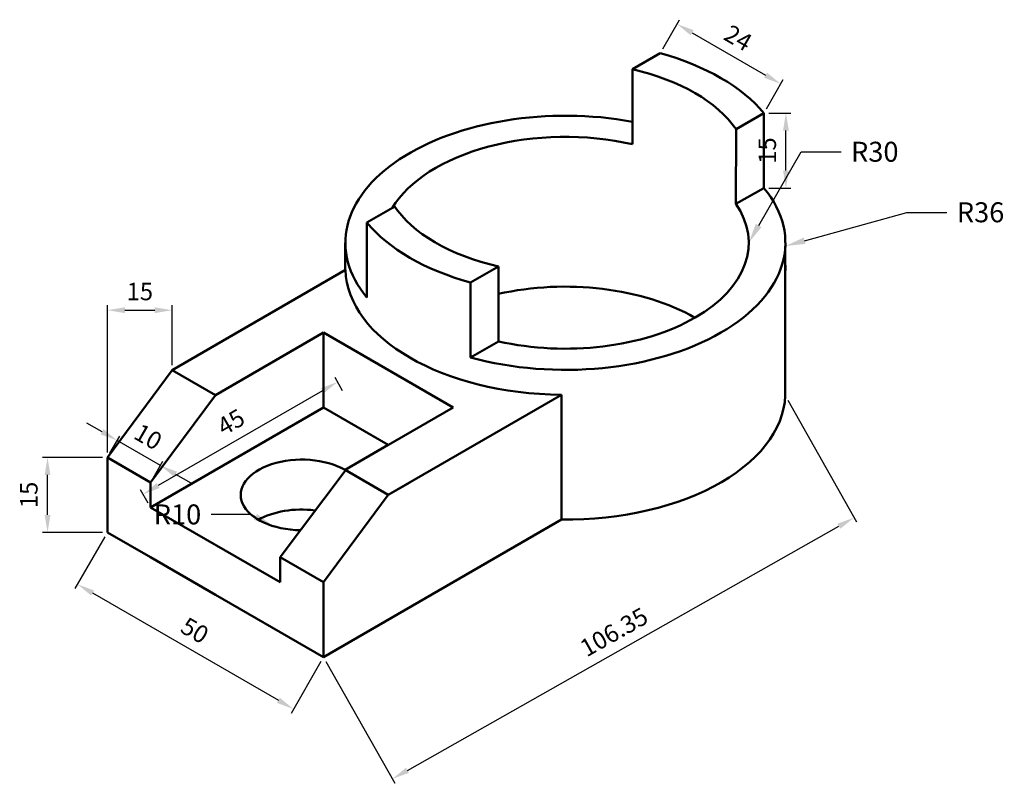
# Model space of a CAD drawing. Units: millimetres. Extents: x 2915 to 3112, y 589 to 742.
import ezdxf
from ezdxf import colors
from ezdxf.entities.mleader import LeaderData, LeaderLine
from ezdxf.math import Vec2, Vec3

# ---------------------------------------------------------------- set-up
doc = ezdxf.new("R2010")
doc.units = ezdxf.units.MM
for name, color, linetype, lineweight in [('M-DIMS', 3, 'Continuous', 25), ('M-OUTL', 7, 'Continuous', 50), ('M-TEXT', 3, 'Continuous', 25)]:
    doc.layers.add(name, color=color, linetype=linetype, lineweight=lineweight)
doc.styles.get("Standard").update_dxf_attribs({"font": 'arial.ttf'})
doc.dimstyles.new('AM_ISO$0', dxfattribs={"dimtxt": 3.5, "dimasz": 3.5, "dimexe": 1, "dimexo": 1, "dimgap": 1.5, "dimtad": 1, "dimdsep": 46, "dimtxsty": 'Standard', "dimcen": 0, "dimclrd": 256, "dimclre": 256, "dimclrt": 2, "dimadec": 0, "dimazin": 2, "dimtp": 0.1, "dimtm": 0.1, "dimtfac": 0.71, "dimtdec": 3, "dimtmove": 0, "dimatfit": 3, "dimfxl": 1, "dimlwd": -1, "dimlwe": -1, "dimarcsym": 1})

# ---------------------------------------------------------------- blocks, each defined once
blk = doc.blocks.new('*D3')
at = {"layer": 'Defpoints', "color": 0, "transparency": 16777216}
for p in [(3064.19, 723.02), (3068.6, 723.02), (3064.19, 708.02)]:
    blk.add_point(p, dxfattribs=at)
at = {"layer": 'M-DIMS', "color": 0, "linetype": 'ByBlock', "transparency": 16777216}
for p, q in [((3065.19, 723.02), (3069.6, 723.02)), ((3068.6, 711.52), (3068.6, 719.52)), ((3065.19, 708.02), (3069.6, 708.02))]:
    blk.add_line(p, q, dxfattribs=at)
at = {"layer": 'M-DIMS', "color": 0, "transparency": 16777216}
for points in [[(3068.02, 719.52), (3069.19, 719.52), (3068.6, 723.02)], [(3068.02, 711.52), (3069.19, 711.52), (3068.6, 708.02)]]:
    blk.add_solid(points, dxfattribs=at)
at = {"layer": 'M-DIMS', "color": 0, "transparency": 16777216, "insert": (3065.32, 715.52), "char_height": 3.5, "attachment_point": 5, "rotation": 90}
blk.add_mtext('15', dxfattribs=at)
blk = doc.blocks.new('*D4')
at = {"layer": 'Defpoints', "color": 0, "transparency": 16777216}
for p in [(3043.4, 735.02), (3067.56, 728.87), (3064.19, 723.02)]:
    blk.add_point(p, dxfattribs=at)
at = {"layer": 'M-DIMS', "color": 0, "linetype": 'ByBlock', "transparency": 16777216}
for p, q in [((3043.9, 735.89), (3047.27, 741.73)), ((3049.81, 739.12), (3064.53, 730.62)), ((3064.69, 723.89), (3068.06, 729.73))]:
    blk.add_line(p, q, dxfattribs=at)
at = {"layer": 'M-DIMS', "color": 0, "transparency": 16777216}
for points in [[(3050.1, 739.62), (3049.51, 738.61), (3046.77, 740.87)], [(3064.82, 731.12), (3064.24, 730.11), (3067.56, 728.87)]]:
    blk.add_solid(points, dxfattribs=at)
at = {"layer": 'M-DIMS', "color": 0, "transparency": 16777216, "insert": (3058.8, 737.69), "char_height": 3.5, "attachment_point": 5, "rotation": 330}
blk.add_mtext('24', dxfattribs=at)
blk = doc.blocks.new('*D5')
at = {"layer": 'Defpoints', "color": 0, "transparency": 16777216}
for p in [(2920.6, 654.05), (2932.6, 654.05), (2932.6, 639.05)]:
    blk.add_point(p, dxfattribs=at)
at = {"layer": 'M-DIMS', "color": 0, "linetype": 'ByBlock', "transparency": 16777216}
for p, q in [((2931.6, 654.05), (2919.6, 654.05)), ((2920.6, 642.55), (2920.6, 650.55)), ((2931.6, 639.05), (2919.6, 639.05))]:
    blk.add_line(p, q, dxfattribs=at)
at = {"layer": 'M-DIMS', "color": 0, "transparency": 16777216}
for points in [[(2920.02, 650.55), (2921.18, 650.55), (2920.6, 654.05)], [(2920.02, 642.55), (2921.18, 642.55), (2920.6, 639.05)]]:
    blk.add_solid(points, dxfattribs=at)
at = {"layer": 'M-DIMS', "color": 0, "transparency": 16777216, "insert": (2917.31, 646.55), "char_height": 3.5, "attachment_point": 5, "rotation": 90}
blk.add_mtext('15', dxfattribs=at)
blk = doc.blocks.new('*D6')
at = {"layer": 'Defpoints', "color": 0, "transparency": 16777216}
for p in [(2932.6, 639.05), (2975.9, 614.05), (2969.9, 603.66)]:
    blk.add_point(p, dxfattribs=at)
at = {"layer": 'M-DIMS', "color": 0, "linetype": 'ByBlock', "transparency": 16777216}
for p, q in [((2932.1, 638.18), (2926.1, 627.79)), ((2929.63, 626.91), (2966.87, 605.41)), ((2975.4, 613.18), (2969.4, 602.79))]:
    blk.add_line(p, q, dxfattribs=at)
at = {"layer": 'M-DIMS', "color": 0, "transparency": 16777216}
for points in [[(2929.92, 627.41), (2929.34, 626.4), (2926.6, 628.66)], [(2967.16, 605.91), (2966.58, 604.9), (2969.9, 603.66)]]:
    blk.add_solid(points, dxfattribs=at)
at = {"layer": 'M-DIMS', "color": 0, "transparency": 16777216, "insert": (2949.89, 619.01), "char_height": 3.5, "attachment_point": 5, "rotation": 330}
blk.add_mtext('50', dxfattribs=at)
blk = doc.blocks.new('*D7')
at = {"layer": 'Defpoints', "color": 0, "transparency": 16777216}
for p in [(2934.56, 657.45), (2932.6, 654.05), (2941.26, 649.05)]:
    blk.add_point(p, dxfattribs=at)
at = {"layer": 'M-DIMS', "color": 0, "linetype": 'ByBlock', "transparency": 16777216}
for p, q in [((2931.53, 659.2), (2928.5, 660.95)), ((2933.1, 654.92), (2935.06, 658.32)), ((2943.22, 652.45), (2934.56, 657.45)), ((2941.76, 649.92), (2943.72, 653.32)), ((2946.25, 650.7), (2949.29, 648.95))]:
    blk.add_line(p, q, dxfattribs=at)
at = {"layer": 'M-DIMS', "color": 0, "transparency": 16777216}
for points in [[(2931.82, 659.71), (2931.24, 658.69), (2934.56, 657.45)], [(2946.55, 651.21), (2945.96, 650.19), (2943.22, 652.45)]]:
    blk.add_solid(points, dxfattribs=at)
at = {"layer": 'M-DIMS', "color": 0, "transparency": 16777216, "insert": (2940.54, 657.8), "char_height": 3.5, "attachment_point": 5, "rotation": 330}
blk.add_mtext('10', dxfattribs=at)
blk = doc.blocks.new('*D8')
at = {"layer": 'Defpoints', "color": 0, "transparency": 16777216}
for p in [(2980.23, 666.55), (2939.75, 646.67), (2941.26, 644.05)]:
    blk.add_point(p, dxfattribs=at)
at = {"layer": 'M-DIMS', "color": 0, "linetype": 'ByBlock', "transparency": 16777216}
for p, q in [((2979.73, 667.42), (2978.22, 670.04)), ((2975.69, 667.42), (2942.78, 648.42)), ((2940.76, 644.92), (2939.25, 647.54))]:
    blk.add_line(p, q, dxfattribs=at)
at = {"layer": 'M-DIMS', "color": 0, "transparency": 16777216}
for points in [[(2975.4, 667.93), (2975.98, 666.92), (2978.72, 669.17)], [(2942.49, 648.93), (2943.07, 647.92), (2939.75, 646.67)]]:
    blk.add_solid(points, dxfattribs=at)
at = {"layer": 'M-DIMS', "color": 0, "transparency": 16777216, "insert": (2957.59, 660.76), "char_height": 3.5, "attachment_point": 5, "rotation": 30}
blk.add_mtext('45', dxfattribs=at)
blk = doc.blocks.new('*D9')
at = {"layer": 'Defpoints', "color": 0, "transparency": 16777216}
for p in [(2945.59, 683.55), (2945.59, 671.55), (2932.6, 654.05)]:
    blk.add_point(p, dxfattribs=at)
at = {"layer": 'M-DIMS', "color": 0, "linetype": 'ByBlock', "transparency": 16777216}
for p, q in [((2932.6, 655.05), (2932.6, 684.55)), ((2936.1, 683.55), (2942.09, 683.55)), ((2945.59, 672.55), (2945.59, 684.55))]:
    blk.add_line(p, q, dxfattribs=at)
at = {"layer": 'M-DIMS', "color": 0, "transparency": 16777216}
for points in [[(2936.1, 684.13), (2936.1, 682.97), (2932.6, 683.55)], [(2942.09, 684.13), (2942.09, 682.97), (2945.59, 683.55)]]:
    blk.add_solid(points, dxfattribs=at)
at = {"layer": 'M-DIMS', "color": 0, "transparency": 16777216, "insert": (2939.1, 686.84), "char_height": 3.5, "attachment_point": 5}
blk.add_mtext('15', dxfattribs=at)
blk = doc.blocks.new('*D10')
at = {"layer": 'Defpoints', "color": 0, "transparency": 16777216}
for p in [(3068.48, 666.39), (3082.27, 642), (2975.9, 614.05)]:
    blk.add_point(p, dxfattribs=at)
at = {"layer": 'M-DIMS', "linetype": 'ByBlock', "transparency": 16777216}
for p, q in [((3068.97, 665.52), (3082.76, 641.13)), ((2992.74, 591.38), (3079.22, 640.28)), ((2976.39, 613.18), (2990.19, 588.79))]:
    blk.add_line(p, q, dxfattribs=at)
at = {"layer": 'M-DIMS', "transparency": 16777216}
for points in [[(3078.93, 640.79), (3079.51, 639.77), (3082.27, 642)], [(2992.45, 591.89), (2993.03, 590.87), (2989.69, 589.66)]]:
    blk.add_solid(points, dxfattribs=at)
at = {"layer": 'M-DIMS', "color": 2, "transparency": 16777216, "insert": (3034.36, 618.69), "char_height": 3.5, "attachment_point": 5, "rotation": 29.4838}
blk.add_mtext('106.35', dxfattribs=at)

msp = doc.modelspace()

# ---------------------------------------------------------------- linework, layer by layer
at = {"layer": 'M-OUTL'}
for p, q in [((3037.819, 731.799), (3043.401, 735.022)), ((3037.819, 731.799), (3037.819, 716.799)), ((3058.603, 719.799), (3064.186, 723.022)), ((3064.186, 723.022), (3064.186, 708.022)), ((3058.603, 719.799), (3058.572, 704.845)), ((3058.572, 704.845), (3064.186, 708.022)), ((2984.613, 701.08), (2990.195, 704.303)), ((2984.613, 701.08), (2984.613, 686.08)), ((2980.255, 691.595), (2980.255, 697.051)), ((3068.475, 696.392), (3068.475, 666.392)), ((2945.591, 671.551), (2980.315, 691.599)), ((3005.398, 689.08), (3010.98, 692.303)), ((3010.98, 692.303), (3010.98, 677.303)), ((3005.398, 689.08), (3005.398, 674.08)), ((2954.251, 666.551), (2975.902, 679.051)), ((2975.902, 679.051), (3001.883, 664.051)), ((2975.902, 679.051), (2975.902, 664.051)), ((3005.398, 674.08), (3010.98, 677.303)), ((2932.601, 654.051), (2945.591, 671.551)), ((2945.591, 671.551), (2954.251, 666.551)), ((2941.261, 649.051), (2954.251, 666.551)), ((2988.892, 646.551), (3023.617, 666.599)), ((3023.617, 641.599), (3023.617, 666.599)), ((2975.902, 664.051), (2941.261, 644.051)), ((2975.902, 664.051), (2988.892, 656.551)), ((3001.883, 664.051), (2980.232, 651.551)), ((2988.892, 656.551), (2980.232, 651.551)), ((2932.601, 639.051), (2932.601, 654.051)), ((2932.601, 654.051), (2941.261, 649.051)), ((2980.232, 651.347), (2967.242, 634.051)), ((2980.232, 651.551), (2988.892, 646.551)), ((2941.261, 649.051), (2941.261, 644.051)), ((2993.222, 649.051), (2988.892, 646.551)), ((2988.892, 646.551), (2975.902, 629.051)), ((2941.261, 644.051), (2967.242, 629.051)), ((2975.902, 614.051), (3023.617, 641.599)), ((2941.261, 634.051), (2932.601, 639.051)), ((2954.251, 626.551), (2941.261, 634.051)), ((2967.242, 634.051), (2975.902, 629.051)), ((2967.242, 634.051), (2967.242, 629.051)), ((2975.902, 629.051), (2975.902, 614.051)), ((2967.242, 619.051), (2954.251, 626.551)), ((2975.902, 614.051), (2967.242, 619.051))]:
    msp.add_line(p, q, dxfattribs=at)
for centre, major_axis, start_param, end_param in [((3024.399, 712.051), (-44.091, 0), 3.5871539, 4.2668277), ((3024.399, 712.051), (-36.742, 0), 3.515474, 4.3385077), ((3024.399, 697.051), (-44.091, 0), 4.4031231, 6.7287466), ((3024.399, 697.051), (-36.742, 0), 4.3385077, 5.948814), ((3024.399, 697.051), (-44.091, 0), 1.1252351, 3.5871539), ((3024.399, 697.051), (-36.742, 0), 1.196915, 3.5178211), ((3024.399, 712.051), (-36.742, 0), 0.3613671, 1.196915), ((3024.399, 712.051), (-44.091, 0), 0.4455613, 1.1252351), ((3024.399, 692.051), (-44.091, 0), 6.3009359, 7.836231), ((3024.399, 692.051), (-44.091, 0), 9.3988883, 9.4506676), ((3024.345, 667.051), (36.742, 0), 0.7853982, 1.9446776), ((3024.399, 667.051), (-44.091, 0), 7.836231, 9.4506676), ((2971.572, 646.551), (-12.247, 0), 3.9269908, 7.8334454), ((2971.518, 636.551), (12.247, 0), 1.352684, 2.3561945)]:
    msp.add_ellipse(centre, major_axis=major_axis, ratio=0.5773503, start_param=start_param, end_param=end_param, dxfattribs=at)

# ---------------------------------------------------------------- dimensions: what is measured, and where the dimension line sits
at = {"layer": 'M-DIMS'}
for p1, p2, distance, override, picture, middle in [((3043.401, 735.022), (3064.186, 723.022), 6.748, {"dimclrd": 0, "dimclre": 0, "dimclrt": 0}, '*D4', (3058.796, 737.686)), ((3064.186, 708.022), (3064.186, 723.022), -4.418, {"dimpost": '', "dimclrd": 0, "dimclre": 0, "dimclrt": 0}, '*D3', (3065.316, 715.522)), ((2980.232, 666.551), (2941.261, 644.051), -3.025, {"dimclrd": 0, "dimclre": 0, "dimclrt": 0}, '*D8', (2957.594, 660.761)), ((2941.261, 649.051), (2932.601, 654.051), -3.925, {"dimclrd": 0, "dimclre": 0, "dimclrt": 0}, '*D7', (2940.537, 657.797)), ((2932.601, 639.051), (2932.601, 654.051), 12, {"dimclrd": 0, "dimclre": 0, "dimclrt": 0}, '*D5', (2917.314, 646.551)), ((2932.601, 639.051), (2975.902, 614.051), -12, {"dimclrd": 0, "dimclre": 0, "dimclrt": 0}, '*D6', (2949.895, 619.005))]:
    dim = msp.add_aligned_dim(p1=p1, p2=p2, distance=distance, dimstyle='AM_ISO$0', override=override, dxfattribs=at)
    dim.commit()
    dim.dimension.update_dxf_attribs({"geometry": picture, "text_midpoint": middle})
dim = msp.add_linear_dim(base=(2945.591, 683.551), p1=(2932.601, 654.051), p2=(2945.591, 671.551), text='15', dimstyle='AM_ISO$0', override={"dimpost": '', "dimclrd": 0, "dimclre": 0, "dimclrt": 0}, dxfattribs=at)
dim.commit()
dim.dimension.update_dxf_attribs({"geometry": '*D9', "text_midpoint": (2939.096, 686.838)})
dim = msp.add_linear_dim(base=(3082.266, 642), p1=(2975.902, 614.051), p2=(3068.475, 666.392), angle=29.48382, dimstyle='AM_ISO$0', override={"dimrnd": 0}, dxfattribs=at)
dim.commit()
dim.dimension.update_dxf_attribs({"geometry": '*D10', "text_midpoint": (3034.361, 618.692)})

# ---------------------------------------------------------------- leaders
at = {"layer": 'M-TEXT'}
ml = msp.add_multileader_mtext('Standard', dxfattribs=at)
ml.set_content('{\\C2;R30}', color=256)
ml.set_leader_properties()
ml.build(insert=Vec2(0, 0))
ctx = ml.context
ctx.base_point, ctx.plane_origin = Vec3(3079.648, 715.248), Vec3(3061.142, 697.051)
notes = []
notes.append((ctx, [(0, (1, 1, 0), (3071.648, 715.248), (1, 0), 8, [(0, [(3061.142, 697.051)], 0, [])])]))
ctx.mtext.insert, ctx.mtext.flow_direction = Vec3(3081.648, 717.283), 5
ml = msp.add_multileader_mtext('Standard', dxfattribs=at)
ml.set_content('{\\C2;R36}', color=256)
ml.set_leader_properties()
ml.build(insert=Vec2(0, 0))
ctx = ml.context
ctx.base_point, ctx.plane_origin = Vec3(3100.853, 703.123), Vec3(3068.475, 696.392)
notes.append((ctx, [(0, (1, 1, 0), (3092.853, 703.123), (1, 0), 8, [(0, [(3068.475, 696.392)], 0, [])])]))
ctx.mtext.insert, ctx.mtext.flow_direction = Vec3(3102.853, 705.158), 5
ml = msp.add_multileader_mtext('Standard', dxfattribs=at)
ml.set_content('{\\C2;R10}', color=256)
ml.set_leader_properties()
ml.build(insert=Vec2(0, 0))
ctx = ml.context
ctx.base_point, ctx.plane_origin = Vec3(2939.862, 642.607), Vec3(2965.82, 640.308)
ctx.text_align_type = 2
notes.append((ctx, [(0, (1, 1, 0), (2961.406, 642.607), (-1, 0), 8, [(0, [(2965.82, 640.308)], 0, [])])]))
ctx.mtext.insert, ctx.mtext.alignment, ctx.mtext.flow_direction = Vec3(2951.406, 644.641), 3, 5
for ctx, leaders in notes:
    for number, flags, end, landing, length, lines in leaders:
        leader = LeaderData()
        leader.index, (leader.has_last_leader_line, leader.has_dogleg_vector, leader.attachment_direction) = number, flags
        leader.last_leader_point, leader.dogleg_vector, leader.dogleg_length = Vec3(end), Vec3(landing), length
        for number, points, colour, breaks in lines:
            line = LeaderLine()
            line.index, line.vertices, line.color, line.breaks = number, Vec3.list(points), colors.encode_raw_color(colour), breaks
            leader.lines.append(line)
        ctx.leaders.append(leader)

doc.saveas('drawing.dxf')
